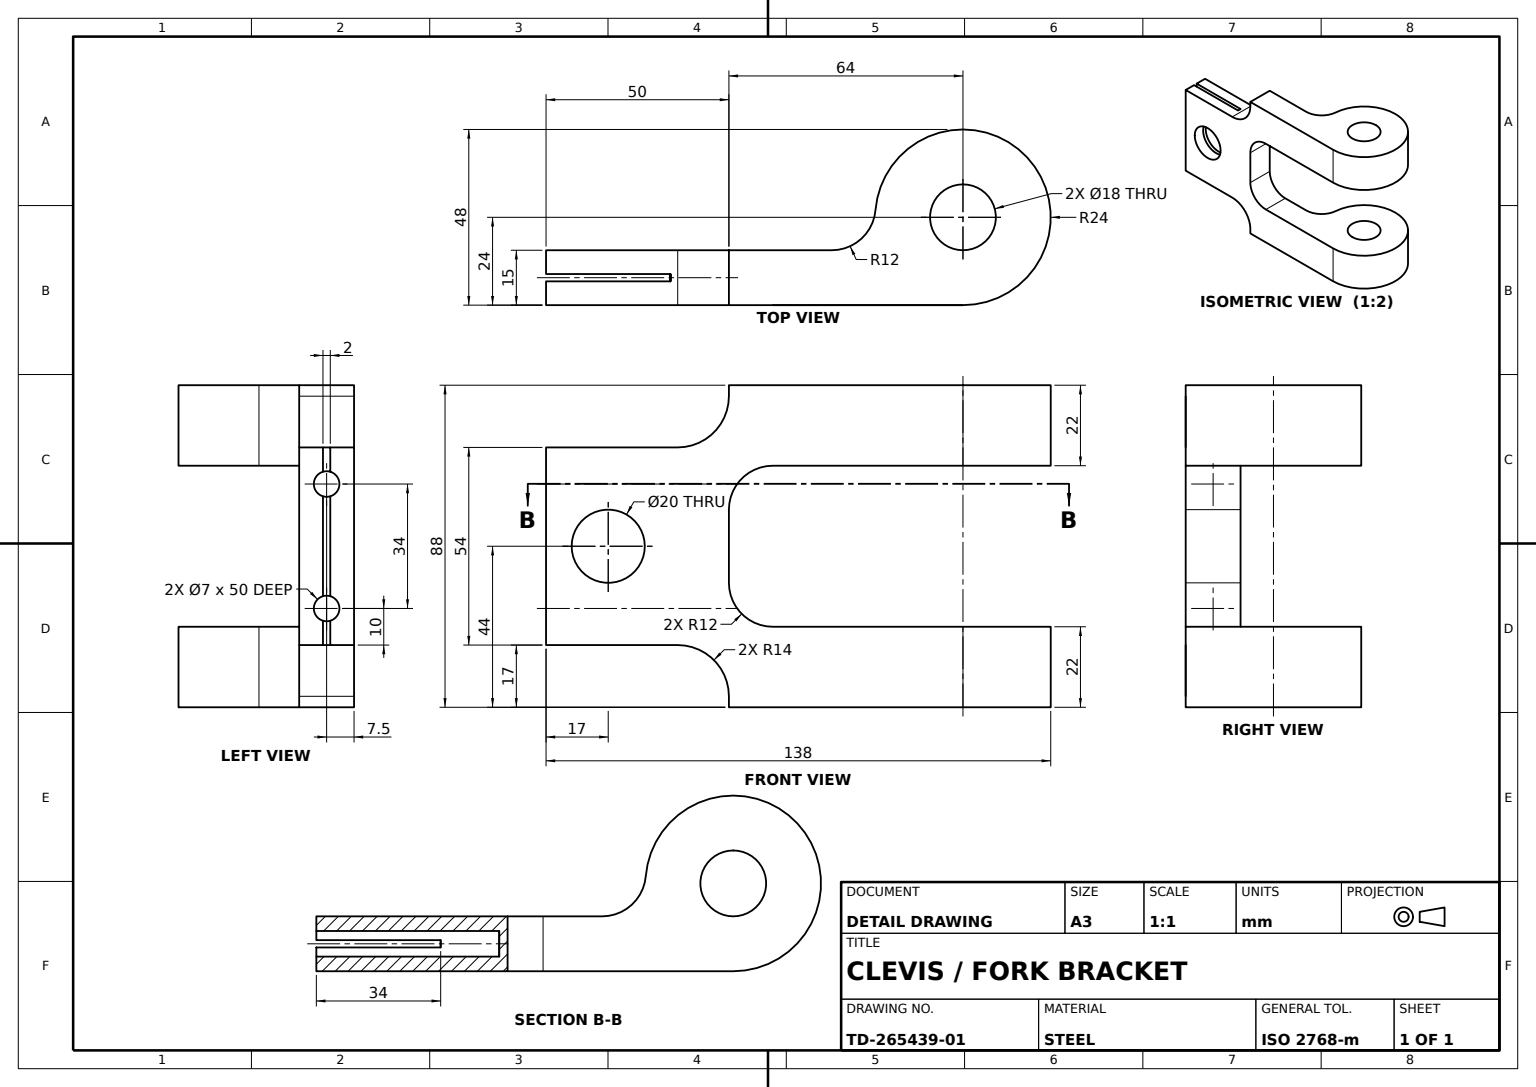
SolidWorks part; units mm, degrees
material "Plain Carbon Steel"
ref_plane "Front Plane" through (0, 0, 0) normal (0, 0, 1) x (1, 0, 0)
ref_plane "Top Plane" through (0, 0, 0) normal (0, 1, 0) x (1, 0, 0)
ref_plane "Right Plane" through (0, 0, 0) normal (1, 0, 0) x (0, 0, -1)
sketch "Fork Body Profile Sketch" plane through (0, 0, 0) normal (0, 1, 0) x (1, 0, 0)
  line L1 (0, -24) -> (-64, -24)
  line L3 (-35.8748, -9) -> (-64, -9)
  line L4 (-64, -24) -> (-64, -9)
  arc A0 (0, -24) -> (-23.9165, 2) centre (0, 0) ccw
  circle A1 centre (0, 0) radius 9
  arc A2 (-23.9165, 2) -> (-35.8748, -9) centre (-35.8748, 3) cw
  dimension "D1" = 48
  dimension "D2" = 18
  dimension "D5" = 12
  dimension "D3" = 15
  dimension "D4" = 64
extrude "Fork Body" add sketch "Fork Body Profile Sketch" along normal mid plane 88
sketch "Offset Tang Sketch" plane through (0, 0, 9) normal (0, 0, -1) x (-1, 0, 0)
  line L0 (64, 44) -> (64, -44) construction
  line L1 (64, 27) -> (114, 27)
  line L2 (64, 27) -> (64, -27)
  line L3 (64, -27) -> (114, -27)
  line L4 (114, 27) -> (114, -27)
  point P6 (114, 0)
  dimension "D1" = 54
  dimension "D2" = 50
extrude "Offset Tang" add sketch "Offset Tang Sketch" against normal up to surface (15 mm away) up to face at (-32, 0, 24)
sketch "Tang Cross Hole Sketch" plane through (0, 0, 9) normal (0, 0, -1) x (-1, 0, 0)
  line L0 (114, -27) -> (114, 27) construction
  circle A0 centre (97, 0) radius 10
  dimension "D1" = 20
  dimension "D2" = 17
extrude "Tang Cross Hole" cut sketch "Tang Cross Hole Sketch" against normal up to next
sketch "Tang Slot Sketch" plane through (0, -27, 0) normal (0, -1, 0) x (1, 0, 0)
  line L0 (-114, 24) -> (-114, 9) construction
  line L1 (-114, 17.5) -> (-80, 17.5)
  line L2 (-114, 17.5) -> (-114, 15.5)
  line L3 (-114, 15.5) -> (-80, 15.5)
  line L4 (-80, 17.5) -> (-80, 15.5)
  line L7 (-64, 24) -> (-64, 9) construction
  point P12 (-64, 16.5)
  point P13 (-80, 16.5)
  dimension "D1" = 2
  dimension "D2" = 34
extrude "Tang Slot 2mm" cut sketch "Tang Slot Sketch" against normal up to next
fillet "Fork Root Fillet R14" radius 14 2 edges at (-64, -27, 16.5) (-64, 27, 16.5)
sketch "Side Relief Sketch" plane through (-114, 0, 0) normal (-1, 0, 0) x (0, 0, 1)
  line L0 (24, 27) -> (17.5, 27) construction
  line L2 (9, -27) -> (9, 27) construction
  line L5 (0, 0) -> (31.1671, 0) construction
  circle A0 centre (16.5, 17) radius 3.5
  circle A1 centre (16.5, -17) radius 3.5
  dimension "D1" = 7
  dimension "D2" = 10
  dimension "D3" = 7.5
extrude "Side Relief Cut" cut sketch "Side Relief Sketch" against normal blind 50
sketch "Fork Eye Profile Sketch" plane through (0, 0, 9) normal (0, 0, -1) x (-1, 0, 0)
  line L0 (35.8748, 44) -> (64, 44) construction
  line L1 (-24, 22) -> (52, 22)
  line L2 (-24, 22) -> (-24, -22)
  line L3 (-24, -22) -> (52, -22)
  line L4 (64, 10) -> (64, -10)
  line L5 (35.8748, -44) -> (64, -44) construction
  line L6 (-24, 44) -> (-24, -44) construction
  arc A0 (52, -22) -> (64, -10) centre (52, -10) ccw
  arc A1 (52, 22) -> (64, 10) centre (52, 10) cw
  point P13 (64, -22)
  dimension "D3" = 12
  dimension "D1" = 22
  dimension "D2" = 22
extrude "Fork Eye Profile Cut" cut sketch "Fork Eye Profile Sketch" against normal through all both and the other way through all
